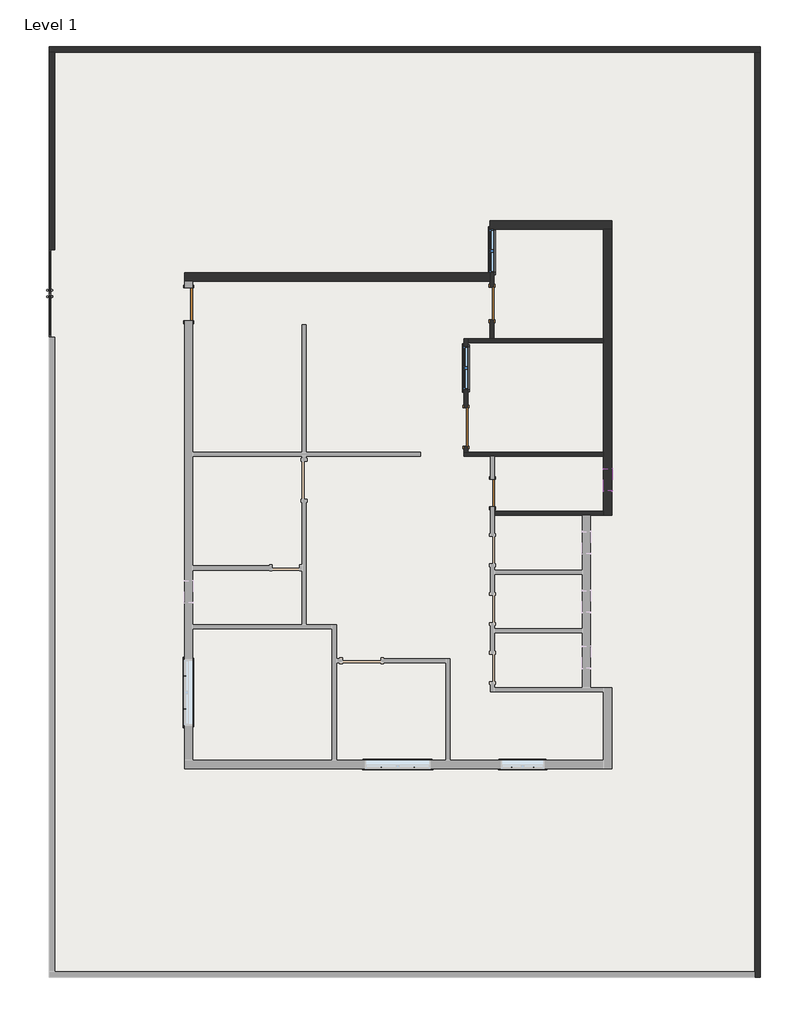
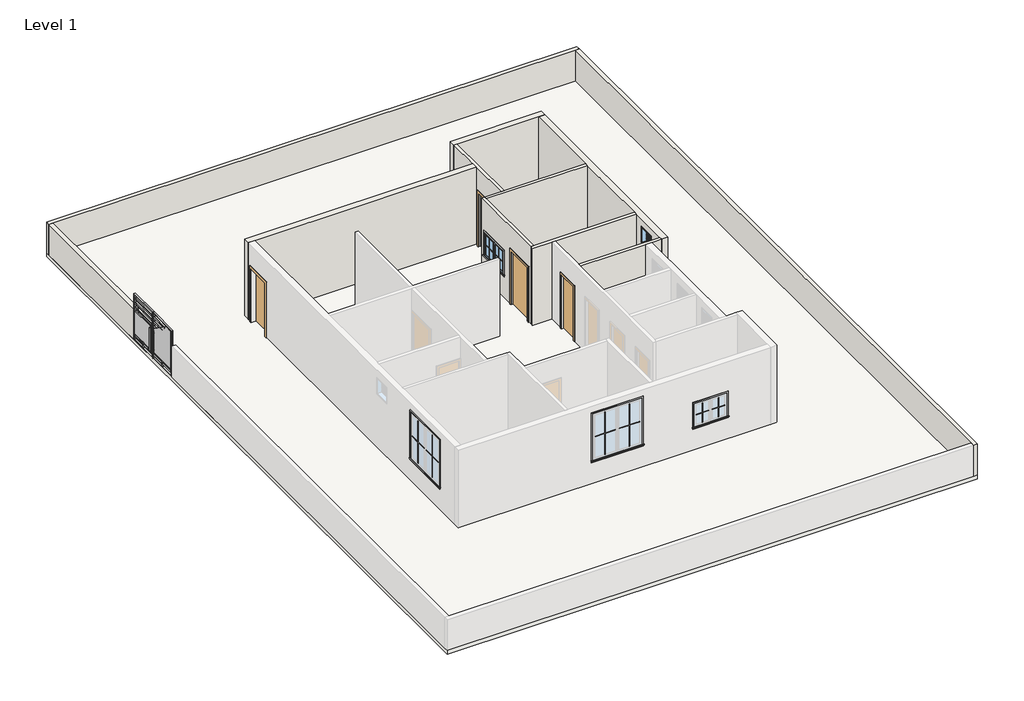
# One storey, part 2 of 2: 21 proxies, 11 walls, 4 doors, 3 windows, 1 slab.
"""IFC4 building model written with IfcOpenShell, lengths in millimetres."""

from ifc_helpers import new_model, si_unit, frame, origin, origin_with_axes, place, context, project, spatial, polyline, outline, extrude, faceted_brep, transform, mapped, element, save
from components import generic_models_113f6068, muntin_pattern_2x2_muntin_pattern_2x2_0a037076, muntin_pattern_2x2_muntin_pattern_2x2_e6f69628, muntin_pattern_2x2_muntin_pattern_2x2_2357e71d, muntin_pattern_2x2_muntin_pattern_2x2_302d8f29, trim_window_exterior_flat_with_sill_b601e94a, trim_window_exterior_flat_with_sill_c4e67c73, trim_window_interior_flat_picture_frame_bfefb25c, trim_window_interior_flat_picture_frame_cf1733af, door_214872d5, single_flush_door_3_305aa2a5, single_flush_door_3_a90ba1ad, door_4c162e62, window_casement_double_win_4_2967420f, window_f2d8fef0

model = new_model("IFC4")

# Units and contexts
model_context = context("Model", 3, world=origin())
ifc_project = project(units=[si_unit("LENGTHUNIT", "METRE", prefix="MILLI")], contexts=[model_context])

# Site, building, storey
site = spatial("IfcSite", under=ifc_project)
building = spatial("IfcBuilding", under=site)
storey = spatial("IfcBuildingStorey", under=building, Name="Level 1", Elevation=0.0)

# Proxies
placement = place(None, origin())
generic_models_shape = generic_models_113f6068(model_context)
element("IfcBuildingElementProxy", 1, Name="Generic Models", at=placement, inside=storey, context=model_context, shape_type="MappedRepresentation", body=[
    mapped(generic_models_shape, transform((-10840.7647743, 6713.245119, 0.0), x_axis=(0.0, 1.0, 0.0), y_axis=(-1.0, 0.0, 0.0), z_axis=(0.0, 0.0, 1.0))),
])
muntin_pattern_2x2_muntin_pattern_2x2_shape = muntin_pattern_2x2_muntin_pattern_2x2_0a037076(model_context)
element("IfcBuildingElementProxy", 2, Name="Muntin Pattern_2x2 : Muntin Pattern_2x2", ObjectType="Muntin Pattern_2x2 : Muntin Pattern_2x2", at=placement, inside=storey, context=model_context, shape_type="MappedRepresentation", body=[
    mapped(muntin_pattern_2x2_muntin_pattern_2x2_shape, transform((-7058.058853, -4848.517381, 984.25), x_axis=(0.0, 1.0, 0.0), y_axis=(-1.0, 0.0, 0.0), z_axis=(0.0, 0.0, 1.0))),
])
element("IfcBuildingElementProxy", 3, Name="Muntin Pattern_2x2 : Muntin Pattern_2x2", ObjectType="Muntin Pattern_2x2 : Muntin Pattern_2x2", at=placement, inside=storey, context=model_context, shape_type="MappedRepresentation", body=[
    mapped(muntin_pattern_2x2_muntin_pattern_2x2_shape, transform((-674.721353, -6497.929881, 984.25), x_axis=(-1.0, 0.0, 0.0), y_axis=(0.0, -1.0, 0.0), z_axis=(0.0, 0.0, 1.0))),
])
muntin_pattern_2x2_muntin_pattern_2x2_2_shape = muntin_pattern_2x2_muntin_pattern_2x2_e6f69628(model_context)
element("IfcBuildingElementProxy", 4, Name="Muntin Pattern_2x2 : Muntin Pattern_2x2", ObjectType="Muntin Pattern_2x2 : Muntin Pattern_2x2", at=placement, inside=storey, context=model_context, shape_type="MappedRepresentation", body=[
    mapped(muntin_pattern_2x2_muntin_pattern_2x2_2_shape, transform((-7058.058853, -3937.292381, 984.25), x_axis=(0.0, -1.0, 0.0), y_axis=(1.0, 0.0, 0.0), z_axis=(0.0, 0.0, 1.0))),
])
element("IfcBuildingElementProxy", 5, Name="Muntin Pattern_2x2 : Muntin Pattern_2x2", ObjectType="Muntin Pattern_2x2 : Muntin Pattern_2x2", at=placement, inside=storey, context=model_context, shape_type="MappedRepresentation", body=[
    mapped(muntin_pattern_2x2_muntin_pattern_2x2_2_shape, transform((-1585.946353, -6497.929881, 984.25), x_axis=(1.0, 0.0, 0.0), y_axis=(0.0, 1.0, 0.0), z_axis=(0.0, 0.0, 1.0))),
])
muntin_pattern_2x2_muntin_pattern_2x2_3_shape = muntin_pattern_2x2_muntin_pattern_2x2_2357e71d(model_context)
element("IfcBuildingElementProxy", 6, Name="Muntin Pattern_2x2 : Muntin Pattern_2x2", ObjectType="Muntin Pattern_2x2 : Muntin Pattern_2x2", at=placement, inside=storey, context=model_context, shape_type="MappedRepresentation", body=[
    mapped(muntin_pattern_2x2_muntin_pattern_2x2_3_shape, transform((2652.678647, -6497.929881, 984.25), x_axis=(-1.0, 0.0, 0.0), y_axis=(0.0, -1.0, 0.0), z_axis=(0.0, 0.0, 1.0))),
])
element("IfcBuildingElementProxy", 7, Name="Muntin Pattern_2x2 : Muntin Pattern_2x2", ObjectType="Muntin Pattern_2x2 : Muntin Pattern_2x2", at=placement, inside=storey, context=model_context, shape_type="MappedRepresentation", body=[
    mapped(muntin_pattern_2x2_muntin_pattern_2x2_3_shape, transform((727.041147, 4333.582619, 984.25), x_axis=(0.0, 1.0, 0.0), y_axis=(-1.0, 0.0, 0.0), z_axis=(0.0, 0.0, 1.0))),
])
element("IfcBuildingElementProxy", 8, Name="Muntin Pattern_2x2 : Muntin Pattern_2x2", ObjectType="Muntin Pattern_2x2 : Muntin Pattern_2x2", at=placement, inside=storey, context=model_context, shape_type="MappedRepresentation", body=[
    mapped(muntin_pattern_2x2_muntin_pattern_2x2_3_shape, transform((1450.941147, 7591.132619, 984.25), x_axis=(0.0, 1.0, 0.0), y_axis=(-1.0, 0.0, 0.0), z_axis=(0.0, 0.0, 1.0))),
])
muntin_pattern_2x2_muntin_pattern_2x2_4_shape = muntin_pattern_2x2_muntin_pattern_2x2_302d8f29(model_context)
element("IfcBuildingElementProxy", 9, Name="Muntin Pattern_2x2 : Muntin Pattern_2x2", ObjectType="Muntin Pattern_2x2 : Muntin Pattern_2x2", at=placement, inside=storey, context=model_context, shape_type="MappedRepresentation", body=[
    mapped(muntin_pattern_2x2_muntin_pattern_2x2_4_shape, transform((2046.253647, -6497.929881, 984.25), x_axis=(1.0, 0.0, 0.0), y_axis=(0.0, 1.0, 0.0), z_axis=(0.0, 0.0, 1.0))),
])
element("IfcBuildingElementProxy", 10, Name="Muntin Pattern_2x2 : Muntin Pattern_2x2", ObjectType="Muntin Pattern_2x2 : Muntin Pattern_2x2", at=placement, inside=storey, context=model_context, shape_type="MappedRepresentation", body=[
    mapped(muntin_pattern_2x2_muntin_pattern_2x2_4_shape, transform((727.041147, 4940.007619, 984.25), x_axis=(0.0, -1.0, 0.0), y_axis=(1.0, 0.0, 0.0), z_axis=(0.0, 0.0, 1.0))),
])
element("IfcBuildingElementProxy", 11, Name="Muntin Pattern_2x2 : Muntin Pattern_2x2", ObjectType="Muntin Pattern_2x2 : Muntin Pattern_2x2", at=placement, inside=storey, context=model_context, shape_type="MappedRepresentation", body=[
    mapped(muntin_pattern_2x2_muntin_pattern_2x2_4_shape, transform((1450.941147, 8197.557619, 984.25), x_axis=(0.0, -1.0, 0.0), y_axis=(1.0, 0.0, 0.0), z_axis=(0.0, 0.0, 1.0))),
])
trim_window_exterior_flat_with_sill_shape = trim_window_exterior_flat_with_sill_b601e94a(model_context)
element("IfcBuildingElementProxy", 12, Name="Trim-Window-Exterior-Flat : with Sill", ObjectType="Trim-Window-Exterior-Flat : with Sill", at=placement, inside=storey, context=model_context, shape_type="MappedRepresentation", body=[
    mapped(trim_window_exterior_flat_with_sill_shape, transform((-7067.583853, -4392.904881, 2743.2), x_axis=(0.0, -1.0, 0.0), y_axis=(0.0, 0.0, 1.0), z_axis=(-1.0, 0.0, 0.0))),
])
element("IfcBuildingElementProxy", 13, Name="Trim-Window-Exterior-Flat : with Sill", ObjectType="Trim-Window-Exterior-Flat : with Sill", at=placement, inside=storey, context=model_context, shape_type="MappedRepresentation", body=[
    mapped(trim_window_exterior_flat_with_sill_shape, transform((-1130.333853, -6507.454881, 2743.2), x_axis=(1.0, 0.0, 0.0), y_axis=(0.0, 0.0, 1.0), z_axis=(0.0, -1.0, 0.0))),
])
trim_window_exterior_flat_with_sill_2_shape = trim_window_exterior_flat_with_sill_c4e67c73(model_context)
element("IfcBuildingElementProxy", 14, Name="Trim-Window-Exterior-Flat : with Sill", ObjectType="Trim-Window-Exterior-Flat : with Sill", at=placement, inside=storey, context=model_context, shape_type="MappedRepresentation", body=[
    mapped(trim_window_exterior_flat_with_sill_2_shape, transform((2349.466147, -6507.454881, 1828.8), x_axis=(1.0, 0.0, 0.0), y_axis=(0.0, 0.0, 1.0), z_axis=(0.0, -1.0, 0.0))),
])
element("IfcBuildingElementProxy", 15, Name="Trim-Window-Exterior-Flat : with Sill", ObjectType="Trim-Window-Exterior-Flat : with Sill", at=placement, inside=storey, context=model_context, shape_type="MappedRepresentation", body=[
    mapped(trim_window_exterior_flat_with_sill_2_shape, transform((717.516147, 4636.795119, 1828.8), x_axis=(0.0, -1.0, 0.0), y_axis=(0.0, 0.0, 1.0), z_axis=(-1.0, 0.0, 0.0))),
])
element("IfcBuildingElementProxy", 16, Name="Trim-Window-Exterior-Flat : with Sill", ObjectType="Trim-Window-Exterior-Flat : with Sill", at=placement, inside=storey, context=model_context, shape_type="MappedRepresentation", body=[
    mapped(trim_window_exterior_flat_with_sill_2_shape, transform((1441.416147, 7894.345119, 1828.8), x_axis=(0.0, -1.0, 0.0), y_axis=(0.0, 0.0, 1.0), z_axis=(-1.0, 0.0, 0.0))),
])
trim_window_interior_flat_picture_frame_shape = trim_window_interior_flat_picture_frame_bfefb25c(model_context)
element("IfcBuildingElementProxy", 17, Name="Trim-Window-Interior-Flat : Picture Frame", ObjectType="Trim-Window-Interior-Flat : Picture Frame", at=placement, inside=storey, context=model_context, shape_type="MappedRepresentation", body=[
    mapped(trim_window_interior_flat_picture_frame_shape, transform((-6838.983853, -4392.904881, 2743.2), x_axis=(0.0, 1.0, 0.0), y_axis=(0.0, 0.0, 1.0), z_axis=(1.0, 0.0, 0.0))),
])
element("IfcBuildingElementProxy", 18, Name="Trim-Window-Interior-Flat : Picture Frame", ObjectType="Trim-Window-Interior-Flat : Picture Frame", at=placement, inside=storey, context=model_context, shape_type="MappedRepresentation", body=[
    mapped(trim_window_interior_flat_picture_frame_shape, transform((-1130.333853, -6278.854881, 2743.2), x_axis=(-1.0, 0.0, 0.0), y_axis=(0.0, 0.0, 1.0), z_axis=(0.0, 1.0, 0.0))),
])
trim_window_interior_flat_picture_frame_2_shape = trim_window_interior_flat_picture_frame_cf1733af(model_context)
element("IfcBuildingElementProxy", 19, Name="Trim-Window-Interior-Flat : Picture Frame", ObjectType="Trim-Window-Interior-Flat : Picture Frame", at=placement, inside=storey, context=model_context, shape_type="MappedRepresentation", body=[
    mapped(trim_window_interior_flat_picture_frame_2_shape, transform((2349.466147, -6278.854881, 1828.8), x_axis=(-1.0, 0.0, 0.0), y_axis=(0.0, 0.0, 1.0), z_axis=(0.0, 1.0, 0.0))),
])
element("IfcBuildingElementProxy", 20, Name="Trim-Window-Interior-Flat : Picture Frame", ObjectType="Trim-Window-Interior-Flat : Picture Frame", at=placement, inside=storey, context=model_context, shape_type="MappedRepresentation", body=[
    mapped(trim_window_interior_flat_picture_frame_2_shape, transform((831.816147, 4636.795119, 1828.8), x_axis=(0.0, 1.0, 0.0), y_axis=(0.0, 0.0, 1.0), z_axis=(1.0, 0.0, 0.0))),
])
element("IfcBuildingElementProxy", 21, Name="Trim-Window-Interior-Flat : Picture Frame", ObjectType="Trim-Window-Interior-Flat : Picture Frame", at=placement, inside=storey, context=model_context, shape_type="MappedRepresentation", body=[
    mapped(trim_window_interior_flat_picture_frame_2_shape, transform((1555.716147, 7894.345119, 1828.8), x_axis=(0.0, 1.0, 0.0), y_axis=(0.0, 0.0, 1.0), z_axis=(1.0, 0.0, 0.0))),
])

# Doors
door_shape = door_214872d5(model_context)
element("IfcDoor", 22, ObjectType="Single-Flush : 2'6\"", at=placement, inside=storey, context=model_context, shape_type="MappedRepresentation", body=[
    mapped(door_shape, transform((1511.266147, 1156.995119, 0.0), x_axis=(0.0, -1.0, 0.0), y_axis=(1.0, 0.0, 0.0), z_axis=(0.0, 0.0, 1.0))),
])
single_flush_door_3_shape = single_flush_door_3_305aa2a5(model_context)
element("IfcDoor", 23, ObjectType="Single-Flush : DOOR 3'", at=placement, inside=storey, context=model_context, shape_type="MappedRepresentation", body=[
    mapped(single_flush_door_3_shape, transform((1498.566147, 6433.845119, 0.0), x_axis=(0.0, 1.0, 0.0), y_axis=(-1.0, 0.0, 0.0), z_axis=(0.0, 0.0, 1.0))),
])
single_flush_door_3_2_shape = single_flush_door_3_a90ba1ad(model_context)
element("IfcDoor", 24, ObjectType="Single-Flush : DOOR 3'", at=placement, inside=storey, context=model_context, shape_type="MappedRepresentation", body=[
    mapped(single_flush_door_3_2_shape, transform((-6953.283853, 6408.445119, 0.0), x_axis=(0.0, 1.0, 0.0), y_axis=(-1.0, 0.0, 0.0), z_axis=(0.0, 0.0, 1.0))),
])
door_2_shape = door_4c162e62(model_context)
element("IfcDoor", 25, ObjectType="Single-Flush : DOOR 3'6\"", at=placement, inside=storey, context=model_context, shape_type="MappedRepresentation", body=[
    mapped(door_2_shape, transform((774.666147, 2998.495119, 0.0), x_axis=(0.0, -1.0, 0.0), y_axis=(1.0, 0.0, 0.0), z_axis=(0.0, 0.0, 1.0))),
])

# Slab
element("IfcSlab", 26, ObjectType="FLOOR 6\"", at=placement, inside=storey, context=model_context, shape_type="SweptSolid", body=[
    extrude(outline(polyline([(-10840.7647743, 13585.4037156), (8971.2352257, 13585.4037156), (8971.2352257, -12322.5962844), (-10840.7647743, -12322.5962844), (-10840.7647743, 13585.4037156)])), frame((0.0, 0.0, -152.4), z_axis=(0.0, 0.0, 1.0), x_axis=(1.0, 0.0, 0.0)), (0.0, 0.0, 1.0), 152.4),
])

# Walls
element("IfcWall", 27, ObjectType="CMD 6\"", at=placement, inside=storey, context=model_context, shape_type="Brep", body=[
    faceted_brep([(-10840.7647743, 13433.0037156, 0.0), (-10688.3647743, 13433.0037156, 0.0), (8818.8352257, 13433.0037156, 0.0), (8971.2352257, 13433.0037156, 0.0), (8971.2352257, 13433.0037156, 1219.2), (8818.8352257, 13433.0037156, 1219.2), (-10688.3647743, 13433.0037156, 1219.2), (-10840.7647743, 13433.0037156, 1219.2), (-10840.7647743, 13585.4037156, 0.0), (-10840.7647743, 13585.4037156, 1219.2), (8971.2352257, 13585.4037156, 1219.2), (8971.2352257, 13585.4037156, 0.0)], [[[0, 1, 2, 3, 4, 5, 6, 7]], [[8, 9, 10, 11]], [[3, 2, 1, 0, 8, 11]], [[7, 6, 5, 4, 10, 9]], [[4, 3, 11, 10]], [[0, 7, 9, 8]]]),
])
element("IfcWall", 28, ObjectType="CMD 6\"", at=placement, inside=storey, context=model_context, shape_type="Brep", body=[
    faceted_brep([(8818.8352257, 13433.0037156, 0.0), (8818.8352257, -12170.1962844, 0.0), (8818.8352257, -12322.5962844, 0.0), (8818.8352257, -12322.5962844, 1219.2), (8818.8352257, -12170.1962844, 1219.2), (8818.8352257, 13433.0037156, 1219.2), (8971.2352257, 13433.0037156, 0.0), (8971.2352257, 13433.0037156, 1219.2), (8971.2352257, -12322.5962844, 1219.2), (8971.2352257, -12322.5962844, 0.0)], [[[0, 1, 2, 3, 4, 5]], [[6, 7, 8, 9]], [[2, 1, 0, 6, 9]], [[5, 4, 3, 8, 7]], [[0, 5, 7, 6]], [[3, 2, 9, 8]]]),
])
element("IfcWall", 29, ObjectType="CMD 6\"", at=placement, inside=storey, context=model_context, shape_type="SweptSolid", body=[
    extrude(outline(polyline([(-10688.3647743, 13433.0037156), (-10688.3647743, 7932.445119), (-10840.7647743, 7932.445119), (-10840.7647743, 13433.0037156), (-10688.3647743, 13433.0037156)])), origin_with_axes(), (0.0, 0.0, 1.0), 1219.2),
])
element("IfcWall", 30, ObjectType="WALL 4.5\"", at=placement, inside=storey, context=model_context, shape_type="Brep", body=[
    faceted_brep([(4603.716147, 2293.645119, 0.0), (831.816147, 2293.645119, 0.0), (717.516147, 2293.645119, 0.0), (717.516147, 2293.645119, 3048.0), (831.816147, 2293.645119, 3048.0), (4603.716147, 2293.645119, 3048.0), (4603.716147, 2179.345119, 0.0), (4603.716147, 2179.345119, 3048.0), (1568.416147, 2179.345119, 3048.0), (1454.116147, 2179.345119, 3048.0), (717.516147, 2179.345119, 3048.0), (717.516147, 2179.345119, 0.0), (1454.116147, 2179.345119, 0.0), (1568.416147, 2179.345119, 0.0)], [[[0, 1, 2, 3, 4, 5]], [[6, 7, 8, 9, 10, 11, 12, 13]], [[2, 1, 0, 6, 13, 12, 11]], [[0, 5, 7, 6]], [[3, 2, 11, 10]], [[5, 4, 3, 10, 9, 8, 7]]]),
])
element("IfcWall", 31, ObjectType="WALL 4.5\"", at=placement, inside=storey, context=model_context, shape_type="Brep", body=[
    faceted_brep([(831.816147, 2293.645119, 0.0), (831.816147, 2465.095119, 0.0), (831.816147, 2465.095119, 2133.6), (831.816147, 3531.895119, 2133.6), (831.816147, 3531.895119, 0.0), (831.816147, 5341.645119, 0.0), (831.816147, 5455.945119, 0.0), (831.816147, 5455.945119, 3048.0), (831.816147, 5341.645119, 3048.0), (831.816147, 2293.645119, 3048.0), (831.816147, 5246.395119, 1828.8), (831.816147, 5246.395119, 914.4), (831.816147, 4027.195119, 914.4), (831.816147, 4027.195119, 1828.8), (717.516147, 2465.095119, 2133.6), (717.516147, 2465.095119, 0.0), (717.516147, 2293.645119, 0.0), (717.516147, 2293.645119, 3048.0), (717.516147, 5455.945119, 3048.0), (717.516147, 5455.945119, 0.0), (717.516147, 3531.895119, 0.0), (717.516147, 3531.895119, 2133.6), (717.516147, 5246.395119, 1828.8), (717.516147, 4027.195119, 1828.8), (717.516147, 4027.195119, 914.4), (717.516147, 5246.395119, 914.4)], [[[0, 1, 2, 3, 4, 5, 6, 7, 8, 9], [10, 11, 12, 13]], [[14, 15, 16, 17, 18, 19, 20, 21], [22, 23, 24, 25]], [[20, 19, 6, 5, 4]], [[16, 15, 1, 0]], [[0, 9, 17, 16]], [[7, 6, 19, 18]], [[11, 10, 22, 25]], [[12, 11, 25, 24]], [[13, 12, 24, 23]], [[10, 13, 23, 22]], [[2, 1, 15, 14]], [[3, 2, 14, 21]], [[4, 3, 21, 20]], [[9, 8, 7, 18, 17]]]),
])
element("IfcWall", 32, ObjectType="WALL 4.5\"", at=placement, inside=storey, context=model_context, shape_type="Brep", body=[
    faceted_brep([(831.816147, 5341.645119, 0.0), (4603.716147, 5341.645119, 0.0), (4603.716147, 5341.645119, 3048.0), (831.816147, 5341.645119, 3048.0), (831.816147, 5455.945119, 0.0), (831.816147, 5455.945119, 3048.0), (1441.416147, 5455.945119, 3048.0), (1555.716147, 5455.945119, 3048.0), (4603.716147, 5455.945119, 3048.0), (4603.716147, 5455.945119, 0.0), (1555.716147, 5455.945119, 0.0), (1441.416147, 5455.945119, 0.0)], [[[0, 1, 2, 3]], [[4, 5, 6, 7, 8, 9, 10, 11]], [[1, 0, 4, 11, 10, 9]], [[0, 3, 5, 4]], [[2, 1, 9, 8]], [[3, 2, 8, 7, 6, 5]]]),
])
element("IfcWall", 33, ObjectType="WALL 4.5\"", at=placement, inside=storey, context=model_context, shape_type="Brep", body=[
    faceted_brep([(1555.716147, 6891.045119, 2133.6), (1555.716147, 6891.045119, 0.0), (1555.716147, 8503.945119, 0.0), (1555.716147, 8503.945119, 914.4), (1555.716147, 7284.745119, 914.4), (1555.716147, 7284.745119, 1828.8), (1555.716147, 8503.945119, 1828.8), (1555.716147, 8503.945119, 3048.0), (1555.716147, 5455.945119, 3048.0), (1555.716147, 5455.945119, 0.0), (1555.716147, 5976.645119, 0.0), (1555.716147, 5976.645119, 2133.6), (1441.416147, 8503.945119, 0.0), (1441.416147, 7284.745119, 0.0), (1441.416147, 7056.145119, 0.0), (1441.416147, 6891.045119, 0.0), (1441.416147, 6891.045119, 2133.6), (1441.416147, 5976.645119, 2133.6), (1441.416147, 5976.645119, 0.0), (1441.416147, 5455.945119, 0.0), (1441.416147, 5455.945119, 3048.0), (1441.416147, 7056.145119, 3048.0), (1441.416147, 7284.745119, 3048.0), (1441.416147, 8503.945119, 3048.0), (1441.416147, 8503.945119, 1828.8), (1441.416147, 7284.745119, 1828.8), (1441.416147, 7284.745119, 914.4), (1441.416147, 8503.945119, 914.4)], [[[0, 1, 2, 3, 4, 5, 6, 7, 8, 9, 10, 11]], [[12, 13, 14, 15, 16, 17, 18, 19, 20, 21, 22, 23, 24, 25, 26, 27]], [[10, 9, 19, 18]], [[2, 1, 15, 14, 13, 12]], [[24, 23, 7, 6]], [[12, 27, 3, 2]], [[9, 8, 20, 19]], [[4, 3, 27, 26]], [[5, 4, 26, 25]], [[6, 5, 25, 24]], [[16, 15, 1, 0]], [[17, 16, 0, 11]], [[18, 17, 11, 10]], [[8, 7, 23, 22, 21, 20]]]),
])
element("IfcWall", 34, ObjectType="WALL 4.5\"", at=placement, inside=storey, context=model_context, shape_type="Brep", body=[
    faceted_brep([(4603.716147, 655.345119, 0.0), (1568.416147, 655.345119, 0.0), (1568.416147, 655.345119, 3048.0), (4603.716147, 655.345119, 3048.0), (4603.716147, 541.045119, 0.0), (4603.716147, 541.045119, 3048.0), (4235.416147, 541.045119, 3048.0), (4006.816147, 541.045119, 3048.0), (1568.416147, 541.045119, 3048.0), (1568.416147, 541.045119, 0.0), (4006.816147, 541.045119, 0.0), (4235.416147, 541.045119, 0.0)], [[[0, 1, 2, 3]], [[4, 5, 6, 7, 8, 9, 10, 11]], [[1, 0, 4, 11, 10, 9]], [[0, 3, 5, 4]], [[2, 1, 9, 8]], [[3, 2, 8, 7, 6, 5]]]),
])
element("IfcWall", 35, ObjectType="WALL 9\"", at=placement, inside=storey, context=model_context, shape_type="Brep", body=[
    faceted_brep([(-7067.583853, 7056.145119, 0.0), (-6838.983853, 7056.145119, 0.0), (1441.416147, 7056.145119, 0.0), (1441.416147, 7056.145119, 3048.0), (-6838.983853, 7056.145119, 3048.0), (-7067.583853, 7056.145119, 3048.0), (-7067.583853, 7284.745119, 0.0), (-7067.583853, 7284.745119, 3048.0), (1441.416147, 7284.745119, 3048.0), (1441.416147, 7284.745119, 0.0)], [[[0, 1, 2, 3, 4, 5]], [[6, 7, 8, 9]], [[2, 1, 0, 6, 9]], [[0, 5, 7, 6]], [[3, 2, 9, 8]], [[5, 4, 3, 8, 7]]]),
])
element("IfcWall", 36, ObjectType="WALL 9\"", at=placement, inside=storey, context=model_context, shape_type="Brep", body=[
    faceted_brep([(1441.416147, 8503.945119, 0.0), (1555.716147, 8503.945119, 0.0), (4603.716147, 8503.945119, 0.0), (4832.316147, 8503.945119, 0.0), (4832.316147, 8503.945119, 3048.0), (4603.716147, 8503.945119, 3048.0), (1555.716147, 8503.945119, 3048.0), (1441.416147, 8503.945119, 3048.0), (1441.416147, 8503.945119, 1828.8), (1441.416147, 8503.945119, 914.4), (1441.416147, 8732.545119, 0.0), (1441.416147, 8732.545119, 3048.0), (4832.316147, 8732.545119, 3048.0), (4832.316147, 8732.545119, 0.0)], [[[0, 1, 2, 3, 4, 5, 6, 7, 8, 9]], [[10, 11, 12, 13]], [[3, 2, 1, 0, 10, 13]], [[4, 3, 13, 12]], [[0, 9, 8, 7, 11, 10]], [[7, 6, 5, 4, 12, 11]]]),
])
element("IfcWall", 37, ObjectType="WALL 9\"", at=placement, inside=storey, context=model_context, shape_type="Brep", body=[
    faceted_brep([(4603.716147, 8503.945119, 0.0), (4603.716147, 5455.945119, 0.0), (4603.716147, 5341.645119, 0.0), (4603.716147, 2293.645119, 0.0), (4603.716147, 2179.345119, 0.0), (4603.716147, 655.345119, 0.0), (4603.716147, 541.045119, 0.0), (4603.716147, 541.045119, 3048.0), (4603.716147, 655.345119, 3048.0), (4603.716147, 2179.345119, 3048.0), (4603.716147, 2293.645119, 3048.0), (4603.716147, 5341.645119, 3048.0), (4603.716147, 5455.945119, 3048.0), (4603.716147, 8503.945119, 3048.0), (4603.716147, 1830.095119, 2743.2), (4603.716147, 1220.495119, 2743.2), (4603.716147, 1220.495119, 2133.6), (4603.716147, 1830.095119, 2133.6), (4832.316147, 8503.945119, 0.0), (4832.316147, 8503.945119, 3048.0), (4832.316147, 541.045119, 3048.0), (4832.316147, 541.045119, 0.0), (4832.316147, 1830.095119, 2743.2), (4832.316147, 1830.095119, 2133.6), (4832.316147, 1220.495119, 2133.6), (4832.316147, 1220.495119, 2743.2)], [[[0, 1, 2, 3, 4, 5, 6, 7, 8, 9, 10, 11, 12, 13], [14, 15, 16, 17]], [[18, 19, 20, 21], [22, 23, 24, 25]], [[6, 5, 4, 3, 2, 1, 0, 18, 21]], [[0, 13, 19, 18]], [[7, 6, 21, 20]], [[23, 22, 14, 17]], [[24, 23, 17, 16]], [[25, 24, 16, 15]], [[22, 25, 15, 14]], [[13, 12, 11, 10, 9, 8, 7, 20, 19]]]),
])

# Windows
window_casement_double_win_4_shape = window_casement_double_win_4_2967420f(model_context)
element("IfcWindow", 38, ObjectType="Window-Casement-Double : WIN 4'", at=placement, inside=storey, context=model_context, shape_type="MappedRepresentation", body=[
    mapped(window_casement_double_win_4_shape, transform((774.666147, 4636.795119, 0.0), x_axis=(0.0, 1.0, 0.0), y_axis=(-1.0, 0.0, 0.0), z_axis=(0.0, 0.0, 1.0))),
])
element("IfcWindow", 39, ObjectType="Window-Casement-Double : WIN 4'", at=placement, inside=storey, context=model_context, shape_type="MappedRepresentation", body=[
    mapped(window_casement_double_win_4_shape, transform((1498.566147, 7894.345119, 0.0), x_axis=(0.0, 1.0, 0.0), y_axis=(-1.0, 0.0, 0.0), z_axis=(0.0, 0.0, 1.0))),
])
window_shape = window_f2d8fef0(model_context)
element("IfcWindow", 40, ObjectType="Window-Louvers : 24\" x 24\"", at=placement, inside=storey, context=model_context, shape_type="MappedRepresentation", body=[
    mapped(window_shape, transform((4724.366147, 1525.295119, 1219.2), x_axis=(0.0, -1.0, 0.0), y_axis=(1.0, 0.0, 0.0), z_axis=(0.0, 0.0, 1.0))),
])

save(model, "model.ifc")

# Revit data of these elements
# Type
#   sheet = none
#   pipe = none
#   handal = none
#   faram = none
#   Default Elevation = 0
# Type "Muntin Pattern_2x2 : Muntin Pattern_2x2"
#   Width [instance default] = 4' - 0"
#   Thickness = 0' - 0 1/2"
#   Height [instance default] = 4' - 0"
#   Distance = 0' - 0 3/4"
#   Interior Material [instance default] = none
#   Exterior Material [instance default] = none
#   Default Elevation = 0
# Type "Trim-Window-Exterior-Flat : with Sill"
#   Trim Width = 0' - 2 1/4"
#   Trim Thickness_Picture Frame = 0' - 1 1/4"
#   Trim Thickness_with Sill = 0' - 0 3/4"
#   Sill Thickness = 0' - 1 1/4"
#   Opening Width [instance default] = 2' - 0"
#   Opening Height [instance default] = 3' - 0"
#   Default Elevation = 4' - 0"
#   Sill = yes
#   Picture Frame = no
#   Trim Material [instance default] = none
# Type "Trim-Window-Interior-Flat : Picture Frame"
#   Trim Thickness_Picture Frame = 0' - 1 1/4"
#   Trim Width = 0' - 2 1/4"
#   Trim Thickness_with Sill = 0' - 0 3/4"
#   Sill Thickness = 0' - 1 1/4"
#   Opening Width [instance default] = 2' - 0"
#   Opening Height [instance default] = 3' - 0"
#   Default Elevation = 4' - 0"
#   Sill = no
#   Picture Frame = yes
#   Trim Material [instance default] = none
# Type "Single-Flush : 2'6\""
#   Type Mark = "10"
#   Construction Type Id = "MDOOR"
#   Assembly Code = "C1020"
#   Analytic Construction = "Metal"
#   Thickness = 0' - 2"
#   Heat Transfer Coefficient (U) = 0.651978 BTU/(h·ft²·°F)
#   Height = 7' - 0"
#   Trim Projection Ext = 0' - 1"
#   Trim Projection Int = 0' - 1"
#   Trim Width = 0' - 3"
#   Width = 2' - 6"
#   Define Thermal Properties by = 1
#   Door Material = Door - Panel
#   Frame Material = Door - Frame
#   Visual Light Transmittance = 0
#   Solar Heat Gain Coefficient = 0
#   Function = (empty or 0)
#   Wall Closure = (empty or 0)
# Type "Single-Flush : DOOR 3'"
#   Type Mark = "8"
#   Construction Type Id = "MDOOR"
#   Assembly Code = "C1020"
#   Analytic Construction = "Metal"
#   Thickness = 0' - 2"
#   Heat Transfer Coefficient (U) = 0.651978 BTU/(h·ft²·°F)
#   Height = 7' - 0"
#   Trim Projection Ext = 0' - 1"
#   Trim Projection Int = 0' - 1"
#   Trim Width = 0' - 3"
#   Width = 3' - 0"
#   Define Thermal Properties by = 1
#   Door Material = Door - Panel
#   Frame Material = Door - Frame
#   Visual Light Transmittance = 0
#   Solar Heat Gain Coefficient = 0
#   Function = (empty or 0)
#   Wall Closure = (empty or 0)
# Type "Single-Flush : DOOR 3'6\""
#   Type Mark = "9"
#   Construction Type Id = "MDOOR"
#   Assembly Code = "C1020"
#   Analytic Construction = "Metal"
#   Thickness = 0' - 2"
#   Heat Transfer Coefficient (U) = 0.651978 BTU/(h·ft²·°F)
#   Height = 7' - 0"
#   Trim Projection Ext = 0' - 1"
#   Trim Projection Int = 0' - 1"
#   Trim Width = 0' - 3"
#   Width = 3' - 6"
#   Define Thermal Properties by = 1
#   Door Material = Door - Panel
#   Frame Material = Door - Frame
#   Visual Light Transmittance = 0
#   Solar Heat Gain Coefficient = 0
#   Function = (empty or 0)
#   Wall Closure = (empty or 0)
# Type "FLOOR 6\""
#   Assembly Code = "B1010"
#   Function = 0
#   Layers, outside or top first: 0' - 6" no material (function 1)
# Type "CMD 6\""
#   Assembly Code = "B2010"
#   Layers, outside or top first: 0' - 6" no material (function 1)
# Type "WALL 4.5\""
#   Assembly Code = "B2010"
#   Layers, outside or top first: 0' - 4 1/2" no material (function 1)
# Type "WALL 9\""
#   Assembly Code = "B2010"
#   Layers, outside or top first: 0' - 9" no material (function 1)
# Type "Window-Casement-Double : WIN 4'"
#   Type Mark = "18"
#   Fire Rating = "0.5h"
#   Assembly Code = "B2020100"
#   Analytic Construction = "Double glazing - domestic"
#   Frame Extension [instance default] = 0' - 0 1/4"
#   Window Inset [instance default] = 0' - 0"
#   Wall Thickness [instance default] = 0' - 6"
#   Interior Wall Closure [instance default] = 0' - 2 1/4"
#   Half Width = 2' - 0"
#   Visual Light Transmittance = 0.81
#   Thermal Resistance (R) = 1.8146 (h·ft²·°F)/BTU
#   Solar Heat Gain Coefficient = 0.76
#   Rough Width = 4' - 0 1/2"
#   Rough Height = 3' - 0 1/2"
#   Height = 3' - 0"
#   Heat Transfer Coefficient (U) = 0.5511 BTU/(h·ft²·°F)
#   Exterior Wall Closure [instance default] = 0' - 1 1/4"
#   Extension Jamb [instance default] = 0' - 2 1/4"
#   Default Sill Height = 3' - 0"
#   Width = 4' - 0"
#   Muntin Visibility = yes
#   Interior Trim Visibility [instance default] = yes
#   Exterior Trim Visibility [instance default] = yes
#   Extension Jamb Visibility [instance default] = yes
#   Interior Trim Material = Wood - Stained
#   Muntin Pattern = Muntin Pattern_2x2 : Muntin Pattern_2x2
#   Interior Trim = Trim-Window-Interior-Flat : Picture Frame
#   Interior Frame Material = Wood - Stained
#   Glass Panel Material = Glass
#   Exterior Trim Material = Clad - White
#   Exterior Trim = Trim-Window-Exterior-Flat : with Sill
#   Exterior Frame Material = Clad - White
#   Wall Closure = (empty or 0)
# Type "Window-Louvers : 24\" x 24\""
#   Type Mark = "20"
#   Construction Type Id = "GSP4R"
#   Assembly Code = "B20"
#   Analytic Construction = "1/8 in Pilkington single glazing"
#   Visual Light Transmittance = 0.9
#   Thermal Resistance (R) = 1.53941 (h·ft²·°F)/BTU
#   Solar Heat Gain Coefficient = 0.78
#   Max Height = 1' - 11.74264"
#   Height = 2' - 0"
#   Heat Transfer Coefficient (U) = 0.6496 BTU/(h·ft²·°F)
#   Blade Width [instance default] = 1' - 10 1/2"
#   Blade Vertical Thickness = 0' - 0.35355"
#   Blade Thickness = 0' - 0 1/4"
#   Blade Spacing = 0' - 1 1/2"
#   Blade Height = 0' - 1.85355"
#   Blade Depth = 0' - 3"
#   Blade Angle = 45.00°
#   Default Sill Height = 3' - 0"
#   Trim Projection_Exterior = 0' - 0 1/2"
#   Trim Projection_Interior = 0' - 0 1/2"
#   Trim Width_Exterior = 0' - 1 1/2"
#   Trim Width_Interior = 0' - 1 1/2"
#   Width = 2' - 0"
#   Max Blade Count = 12
#   Define Thermal Properties by = 1
#   Blade Count = 12
#   Frame Material = Birch
#   Louver Material = Birch
#   Trim Exterior Material = Birch
#   Trim Interior Material = Birch
#   Wall Closure = (empty or 0)
# Element 1 (IfcBuildingElementProxy)
#   Phase Created = New Construction
# Elements 2, 3, 4, 5 (IfcBuildingElementProxy, "Muntin Pattern_2x2 : Muntin Pattern_2x2")
#   Width = 2' - 6 5/8"
#   Height = 5' - 6 1/2"
#   Interior Material = Wood - Stained
#   Exterior Material = Clad - White
#   Phase Created = New Construction
#   Materials on its faces: "Clad - White", "Wood - Stained"
# Elements 6, 7, 8, 9, 10, 11 (IfcBuildingElementProxy, "Muntin Pattern_2x2 : Muntin Pattern_2x2")
#   Width = 1' - 6 5/8"
#   Height = 2' - 6 1/2"
#   Interior Material = Wood - Stained
#   Exterior Material = Clad - White
#   Phase Created = New Construction
#   Materials on its faces: "Clad - White", "Wood - Stained"
# Elements 12, 13 (IfcBuildingElementProxy, "Trim-Window-Exterior-Flat : with Sill")
#   Opening Width = 6' - 0"
#   Opening Height = 6' - 0"
#   Trim Material = Clad - White
#   Phase Created = New Construction
#   Materials on its faces: "Clad - White"
# Elements 14, 15, 16 (IfcBuildingElementProxy, "Trim-Window-Exterior-Flat : with Sill")
#   Opening Width = 4' - 0"
#   Opening Height = 3' - 0"
#   Trim Material = Clad - White
#   Phase Created = New Construction
#   Materials on its faces: "Clad - White"
# Elements 17, 18 (IfcBuildingElementProxy, "Trim-Window-Interior-Flat : Picture Frame")
#   Opening Width = 6' - 0"
#   Opening Height = 6' - 0"
#   Trim Material = Wood - Stained
#   Phase Created = New Construction
#   Materials on its faces: "Wood - Stained"
# Elements 19, 20, 21 (IfcBuildingElementProxy, "Trim-Window-Interior-Flat : Picture Frame")
#   Opening Width = 4' - 0"
#   Opening Height = 3' - 0"
#   Trim Material = Wood - Stained
#   Phase Created = New Construction
#   Materials on its faces: "Wood - Stained"
# Element 22 (IfcDoor, "Single-Flush : 2'6\"")
#   Phase Created = New Construction
#   Materials on its faces: "Door - Frame", "Door - Panel"
# Elements 23, 24 (IfcDoor, "Single-Flush : DOOR 3'")
#   Phase Created = New Construction
#   Materials on its faces: "Door - Frame", "Door - Panel"
# Element 25 (IfcDoor, "Single-Flush : DOOR 3'6\"")
#   Phase Created = New Construction
#   Materials on its faces: "Door - Frame", "Door - Panel"
# Element 26 (IfcSlab, "FLOOR 6\"")
#   built-in parameter 1001955 = 3.14159 (stored number, unit not read)
#   Height Offset From Level = 0' - 0"
#   Phase Created = New Construction
#   Materials on its faces: "Default Floor", "Wood Planks"
# Elements 27, 29 (IfcWall, "CMD 6\"")
#   Top Offset = 0' - 0"
#   Base Offset = 0' - 0"
#   Unconnected Height = 4' - 0"
#   wall height = 4' - 0"
#   Phase Created = New Construction
#   Base Constraint = Level 1
#   Materials on its faces: "Default Wall", "Clad - White", "Wood - Stained"
# Element 28 (IfcWall, "CMD 6\"")
#   Top Offset = 0' - 0"
#   Base Offset = 0' - 0"
#   Unconnected Height = 4' - 0"
#   wall height = 4' - 0"
#   Phase Created = New Construction
#   Base Constraint = Level 1
#   Materials on its faces: "Default Wall", "Clad - White"
# Elements 30, 31, 32 (IfcWall, "WALL 4.5\"")
#   Top Offset = 0' - 0"
#   Base Offset = 0' - 0"
#   Unconnected Height = 10' - 0"
#   wall height = 10' - 0"
#   Phase Created = New Construction
#   Base Constraint = Level 1
#   Materials on its faces: "Default Wall"
# Elements 33, 34 (IfcWall, "WALL 4.5\"")
#   Top Offset = 0' - 0"
#   Base Offset = 0' - 0"
#   Unconnected Height = 10' - 0"
#   wall height = 10' - 0"
#   Phase Created = New Construction
#   Base Constraint = Level 1
#   Materials on its faces: "Default Wall", "Wood - Stained"
# Elements 35, 36, 37 (IfcWall, "WALL 9\"")
#   Top Offset = 0' - 0"
#   Base Offset = 0' - 0"
#   Unconnected Height = 10' - 0"
#   wall height = 10' - 0"
#   Phase Created = New Construction
#   Base Constraint = Level 1
#   Materials on its faces: "Default Wall", "Wood - Stained"
# Element 38 (IfcWindow, "Window-Casement-Double : WIN 4'")
#   Mark = "4"
#   Window Inset = 0' - 0"
#   Interior Wall Closure = 0' - 2 1/4"
#   Frame Extension = 0' - 0 1/4"
#   Exterior Wall Closure = 0' - 1 1/4"
#   Interior Trim Visibility = yes
#   Exterior Trim Visibility = yes
#   Phase Created = New Construction
#   Materials on its faces: "Wood - Stained", "Glass", "Clad - White"
# Element 39 (IfcWindow, "Window-Casement-Double : WIN 4'")
#   Mark = "5"
#   Window Inset = 0' - 0"
#   Interior Wall Closure = 0' - 2 1/4"
#   Frame Extension = 0' - 0 1/4"
#   Exterior Wall Closure = 0' - 1 1/4"
#   Interior Trim Visibility = yes
#   Exterior Trim Visibility = yes
#   Phase Created = New Construction
#   Materials on its faces: "Wood - Stained", "Glass", "Clad - White"
# Element 40 (IfcWindow, "Window-Louvers : 24\" x 24\"")
#   Mark = "6"
#   Blade Width = 1' - 10 1/2"
#   Phase Created = New Construction
#   Materials on its faces: "Birch"
# Materials
#   "Door - Panel": class "Wood", colour RGB 210 159 95, transparency 0, Cost = 0
#   "Door - Frame": colour RGB 118 70 51, transparency 0, Cost = 0
#   "Wood - Stained": class "Wood", colour RGB 224 178 126, transparency 0, Cost = 0
#   "Glass": class "Glass", colour RGB 0 128 192, transparency 0.75, Description = "Soda Lime Glass", Cost = 0
#   "Clad - White": class "Wood", colour RGB 242 242 238, transparency 0, Cost = 0
#   "Birch": class "Wood", colour RGB 224 178 126, transparency 0, Description = "Betula Alleghaniensis", Cost = 0
#   "Default Floor": colour RGB 128 128 128, transparency 0, Cost = 0
#   "Wood Planks": class "Wood", colour RGB 193 160 115, transparency 0, Description = "Physical material.", Cost = 0
#   "Default Wall": colour RGB 128 128 128, transparency 0, Cost = 0
